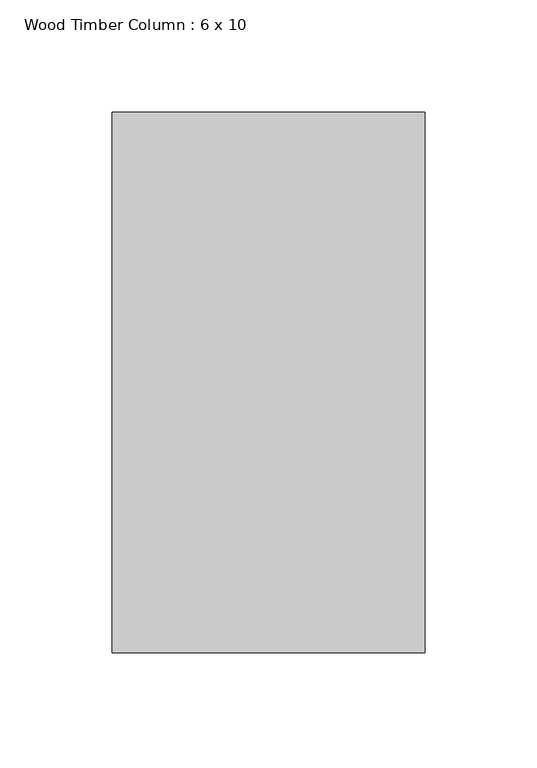
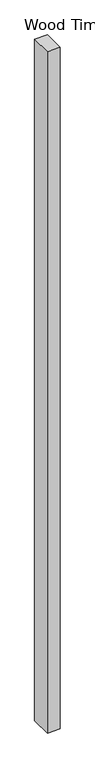
"""IFC4 building model written with IfcOpenShell, lengths in millimetres: column geometry, Wood Timber Column : 6 x 10."""

from ifc_helpers import new_model, si_unit, frame, origin, place, context, project, spatial, polyline, outline, extrude, source, transform, mapped, element, save


def wood_timber_column_6_x_10_a3b0a8a3(model_context):
    return source(origin(), model_context, "Body", "SweptSolid", [
        extrude(outline(polyline([(69.85, -120.65), (-69.85, -120.65), (-69.85, 120.65), (69.85, 120.65), (69.85, -120.65)])), frame((0.0, 0.0, 7931.15), z_axis=(0.0, 0.0, 1.0), x_axis=(1.0, 0.0, 0.0)), (0.0, 0.0, 1.0), 7924.8),
    ])


if __name__ == "__main__":
    model = new_model("IFC4")
    model_context = context("Model", 3, world=origin())
    ifc_project = project(units=[si_unit("LENGTHUNIT", "METRE", prefix="MILLI")], contexts=[model_context])
    site = spatial("IfcSite", under=ifc_project)
    building = spatial("IfcBuilding", under=site)
    placement = place(None, origin())
    wood_timber_column_6_x_10_shape = wood_timber_column_6_x_10_a3b0a8a3(model_context)
    element("IfcColumn", 1, ObjectType="Wood Timber Column : 6 x 10", at=placement, inside=building, context=model_context, shape_type="MappedRepresentation", body=[
        mapped(wood_timber_column_6_x_10_shape, transform((0.0, 0.0, 0.0), x_axis=(1.0, 0.0, 0.0), y_axis=(0.0, 1.0, 0.0), z_axis=(0.0, 0.0, 1.0))),
    ])
    save(model, "model.ifc")

# Revit data of these elements
# Type "Wood Timber Column : 6 x 10"
#   Assembly Code = "B1010200"
#   Depth = 0' - 9 1/2"
#   Width = 0' - 5 1/2"
#   Material = Softwood, Lumber
# Element 1 (IfcColumn, "Wood Timber Column : 6 x 10")
#   Materials on its faces: "Softwood, Lumber"
# Materials
#   "Softwood, Lumber": class "Wood", colour RGB 223 192 134, transparency 0, Description = "Pinus Echinata", Cost = 0
